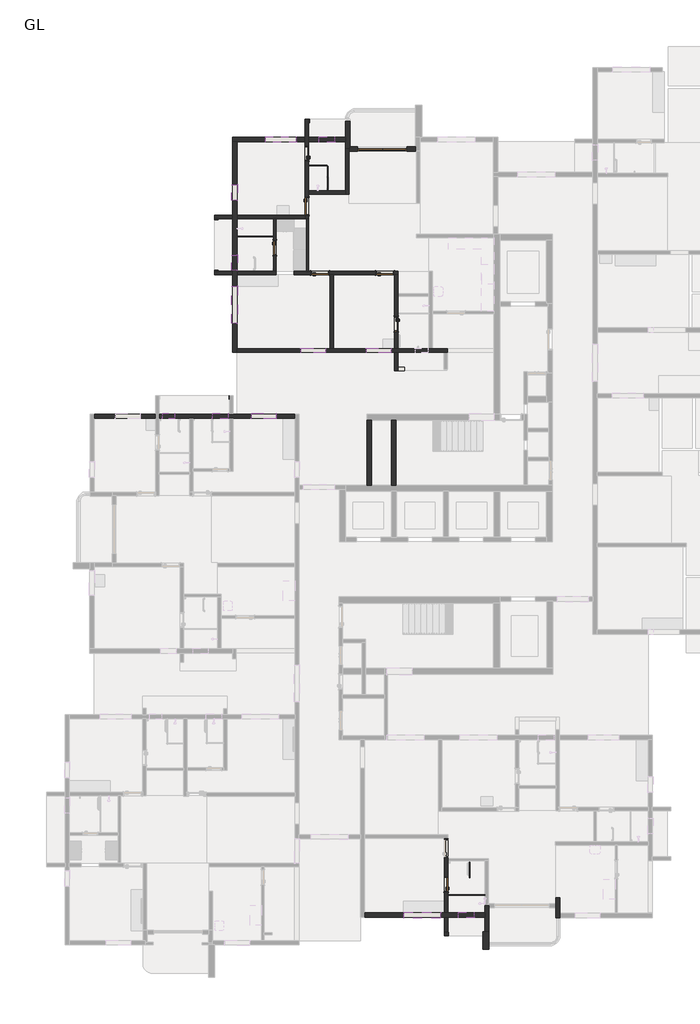
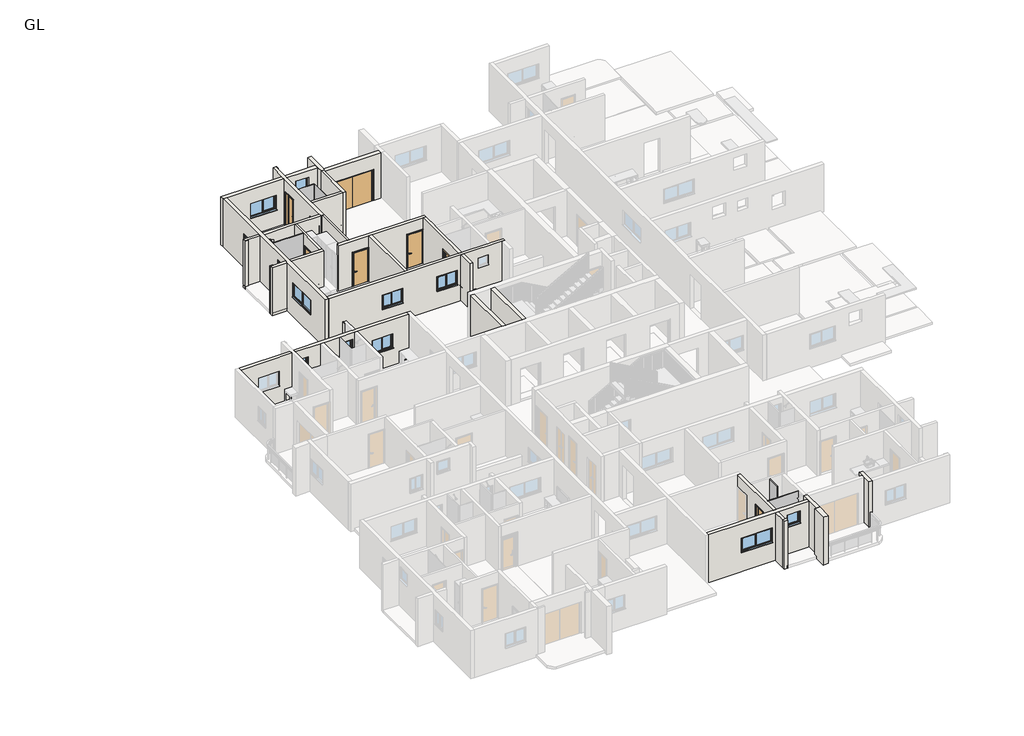
# One storey, part 3 of 14: 30 walls, 12 windows, 8 doors, 5 plates.
# Revit data of these elements (continued)
# Type "Windows_Dbl_Plain : 6'" (continued)
#   Heat Transfer Coefficient (U) = 3.6886 W/(m²·K)
#   Glazing Thickness = 0.07874 ft
#   FrameOffset - External = 0.164042 ft
#   Frame Depth = 0.213255 ft
#   Default Head Height = 6.922572 ft
#   Cill Depth = 0.287073 ft
#   Cavity Closer Width = 0.164042 ft
#   Cavity Closer Offset from Ext = 0.336286 ft
#   Cavity Closer Depth = 0.278871 ft
#   Vis - Cavity Closers = yes
#   Define Thermal Properties by = 1
#   Material Trim = Window Frame
#   Material Glass = Glass
#   Material Frame = Window Frame
#   Wall Closure = (empty or 0)
# Type "Windows_Sgl_Plain : 2'"
#   Type Mark = "60"
#   Operation = "SinglePanel"
#   Construction Type Id = "SGL"
#   Manufacturer = "Revit"
#   Keynote = "L10"
#   Analytic Construction = "Large single-glazed windows"
#   Wrap Layers (Ext) from Ext = 0.336286 ft
#   Wrap Layers (Int) from Ext = 0.582349 ft
#   Window Board Projection = 0.082021 ft
#   Window Board Extension = 0.082021 ft
#   Visual Light Transmittance = 0.9
#   Solar Heat Gain Coefficient = 0.86
#   Rough Width = 2.0 ft
#   Rough Height = 2.0 ft
#   Height = 2.0 ft
#   Width = 2.0 ft
#   Heat Transfer Coefficient (U) = 5.5617 W/(m²·K)
#   Glazing Thickness = 0.07874 ft
#   FrameOffset - External = 0.164042 ft
#   Frame Depth = 0.213255 ft
#   Default Head Height = 6.922572 ft
#   Cill Depth = 0.287073 ft
#   Cavity Closer Width = 0.164042 ft
#   Cavity Closer Offset from Ext = 0.336286 ft
#   Cavity Closer Depth = 0.278871 ft
#   Vis - Cavity Closers = yes
#   Define Thermal Properties by = 1
#   Material Trim = Window Frame
#   Material Glass = Glass
#   Material Frame = Window Frame
#   Wall Closure = (empty or 0)
# Type "Windows_Sgl_Plain : 2.5'"
#   Type Mark = "61"
#   Operation = "SinglePanel"
#   Construction Type Id = "SGL"
#   Manufacturer = "Revit"
#   Keynote = "L10"
#   Analytic Construction = "Large single-glazed windows"
#   Wrap Layers (Ext) from Ext = 0.336286 ft
#   Wrap Layers (Int) from Ext = 0.582349 ft
#   Window Board Projection = 0.082021 ft
#   Window Board Extension = 0.082021 ft
#   Visual Light Transmittance = 0.9
#   Solar Heat Gain Coefficient = 0.86
#   Rough Width = 2.5 ft
#   Rough Height = 2.5 ft
#   Height = 2.5 ft
#   Width = 2.5 ft
#   Heat Transfer Coefficient (U) = 5.5617 W/(m²·K)
#   Glazing Thickness = 0.07874 ft
#   FrameOffset - External = 0.164042 ft
#   Frame Depth = 0.213255 ft
#   Default Head Height = 6.922572 ft
#   Cill Depth = 0.287073 ft
#   Cavity Closer Width = 0.164042 ft
#   Cavity Closer Offset from Ext = 0.336286 ft
#   Cavity Closer Depth = 0.278871 ft
#   Vis - Cavity Closers = yes
#   Define Thermal Properties by = 1
#   Material Trim = Window Frame
#   Material Glass = Glass
#   Material Frame = Window Frame
#   Wall Closure = (empty or 0)
# Element 1 (IfcDoor, "Doors_Concept_ExtDbl : 8'")
#   Phase Created = New Construction
#   Materials on its faces: "Concept", "Door - Glazing"
# Elements 2, 3, 4, 5 (IfcDoor, "Doors_IntSgl : 2.5' DOOR")
#   Phase Created = New Construction
#   Materials on its faces: "Door - Architrave", "Door - Handle", "Door - Frame/Mullion (1)", "Door - Panel"
# Elements 6, 7, 8 (IfcDoor, "Doors_IntSgl : 3' DOOR")
#   Phase Created = New Construction
#   Materials on its faces: "Door - Architrave", "Door - Handle", "Door - Frame/Mullion (1)", "Door - Panel"
# Elements 9, 10, 11, 12, 13 (IfcPlate, "System Panel : Glazed")
#   Phase Created = New Construction
#   Materials on its faces: "Glass"
# Elements 14, 15, 16, 17, 18, 19, 20, 21, 22, 23, 24, 25, 27, 28, 29 (IfcWall, "W2")
#   Top Offset = 0.0 ft
#   Base Offset = 0.0 ft
#   wall height = 9.84252 ft
#   Phase Created = New Construction
#   Base Constraint = GL
#   Top Constraint = FFL
#   Materials on its faces: "Brick, Common"
# Element 26 (IfcWall, "W2")
#   Top Offset = -6.0 ft
#   Base Offset = 0.0 ft
#   wall height = 3.84252 ft
#   Phase Created = New Construction
#   Base Constraint = GL
#   Top Constraint = FFL
#   Materials on its faces: "Brick, Common"
# Elements 30, 31 (IfcWall, "W3")
#   Top Offset = 0.0 ft
#   Base Offset = 0.0 ft
#   wall height = 9.84252 ft
#   Phase Created = New Construction
#   Base Constraint = GL
#   Top Constraint = FFL
#   Materials on its faces: "Brick, Common"
# Element 32 (IfcWall, "W4")
#   Top Offset = 0.0 ft
#   Base Offset = 0.0 ft
#   wall height = 9.84252 ft
#   Phase Created = New Construction
#   Base Constraint = GL
#   Top Constraint = FFL
#   Materials on its faces: "Brick, Common"
# Elements 33, 34, 35 (IfcWall, "W5")
#   Top Offset = 0.0 ft
#   Base Offset = 0.0 ft
#   wall height = 9.84252 ft
#   Phase Created = New Construction
#   Base Constraint = GL
#   Top Constraint = FFL
#   Materials on its faces: "Brick, Common"
# Elements 36, 37 (IfcWall, "W7")
#   Top Offset = 0.0 ft
#   Base Offset = 0.0 ft
#   wall height = 9.84252 ft
#   Phase Created = New Construction
#   Base Constraint = GL
#   Top Constraint = FFL
#   Materials on its faces: "Brick, Common"
# Elements 38, 39, 40, 41 (IfcWall, "W8")
#   Top Offset = 0.0 ft
#   Base Offset = 0.0 ft
#   wall height = 9.84252 ft
#   Phase Created = New Construction
#   Base Constraint = GL
#   Top Constraint = FFL
#   Materials on its faces: "Brick, Common"
# Element 42 (IfcWall, "W9")
#   Top Offset = 0.0 ft
#   Base Offset = 0.0 ft
#   wall height = 9.84252 ft
#   Phase Created = New Construction
#   Base Constraint = GL
#   Top Constraint = FFL
#   Materials on its faces: "Brick, Common"
# Element 43 (IfcWall, "WALL 1")
#   Top Offset = 0.0 ft
#   Base Offset = 0.0 ft
#   wall height = 9.84252 ft
#   Phase Created = New Construction
#   Base Constraint = GL
#   Top Constraint = FFL
#   Materials on its faces: "Brick, Common"
# Element 44 (IfcWindow, "Windows_Dbl_Plain : 2.5'")
#   Mark = "51"
#   Phase Created = New Construction
#   Materials on its faces: "Window Frame", "Glass"
# Element 45 (IfcWindow, "Windows_Dbl_Plain : 4'")
#   Mark = "66"
#   Phase Created = New Construction
#   Materials on its faces: "Window Frame", "Glass"
# Element 46 (IfcWindow, "Windows_Dbl_Plain : 4'")
#   Mark = "54"
#   Phase Created = New Construction
#   Materials on its faces: "Window Frame", "Glass"
# Element 47 (IfcWindow, "Windows_Dbl_Plain : 4'")
#   Mark = "55"
#   Phase Created = New Construction
#   Materials on its faces: "Window Frame", "Glass"
# Element 48 (IfcWindow, "Windows_Dbl_Plain : 5'")
#   Mark = "50"
#   Phase Created = New Construction
#   Materials on its faces: "Window Frame", "Glass"
# Element 49 (IfcWindow, "Windows_Dbl_Plain : 6'")
#   Mark = "14"
#   Phase Created = New Construction
#   Materials on its faces: "Window Frame", "Glass"
# Element 50 (IfcWindow, "Windows_Dbl_Plain : 6'")
#   Mark = "53"
#   Phase Created = New Construction
#   Materials on its faces: "Window Frame", "Glass"
# Element 51 (IfcWindow, "Windows_Sgl_Plain : 2'")
#   Mark = "64"
#   Phase Created = New Construction
#   Materials on its faces: "Window Frame", "Glass"
# Element 52 (IfcWindow, "Windows_Sgl_Plain : 2.5'")
#   Mark = "65"
#   Phase Created = New Construction
#   Materials on its faces: "Window Frame", "Glass"
# Element 53 (IfcWindow, "Windows_Sgl_Plain : 2.5'")
#   Mark = "15"
#   Phase Created = New Construction
#   Materials on its faces: "Window Frame", "Glass"
# Element 54 (IfcWindow, "Windows_Sgl_Plain : 2.5'")
#   Mark = "49"
#   Phase Created = New Construction
#   Materials on its faces: "Window Frame", "Glass"
# Element 55 (IfcWindow, "Windows_Sgl_Plain : 2.5'")
#   Mark = "52"
#   Phase Created = New Construction
#   Materials on its faces: "Window Frame", "Glass"
# Materials
#   "Door - Glazing": colour RGB 0 0 255, transparency 0.75
#   "Concept": colour RGB 128 128 255, transparency 0.5
#   "Door - Handle": colour RGB 0 0 0, transparency 0, Keynote = "P21", Cost = 0
#   "Door - Frame/Mullion (1)": class "Wood", colour RGB 212 179 113, transparency 0, Keynote = "L20", Cost = 0
#   "Door - Panel": class "Wood", colour RGB 210 159 95, transparency 0, Keynote = "L20", Cost = 0
#   "Door - Architrave": class "Wood", colour RGB 154 90 5, transparency 0, Keynote = "P20", Cost = 0
#   "Brick, Common": class "Masonry", colour RGB 170 100 105, transparency 0, Description = "Common brick", Cost = 0
#   "Window Frame": colour RGB 249 249 249, transparency 0, Keynote = "L10", Cost = 0
#   "Glass": class "Glass", colour RGB 0 128 192, transparency 0.9, Description = "Soda Lime Glass", Cost = 0
